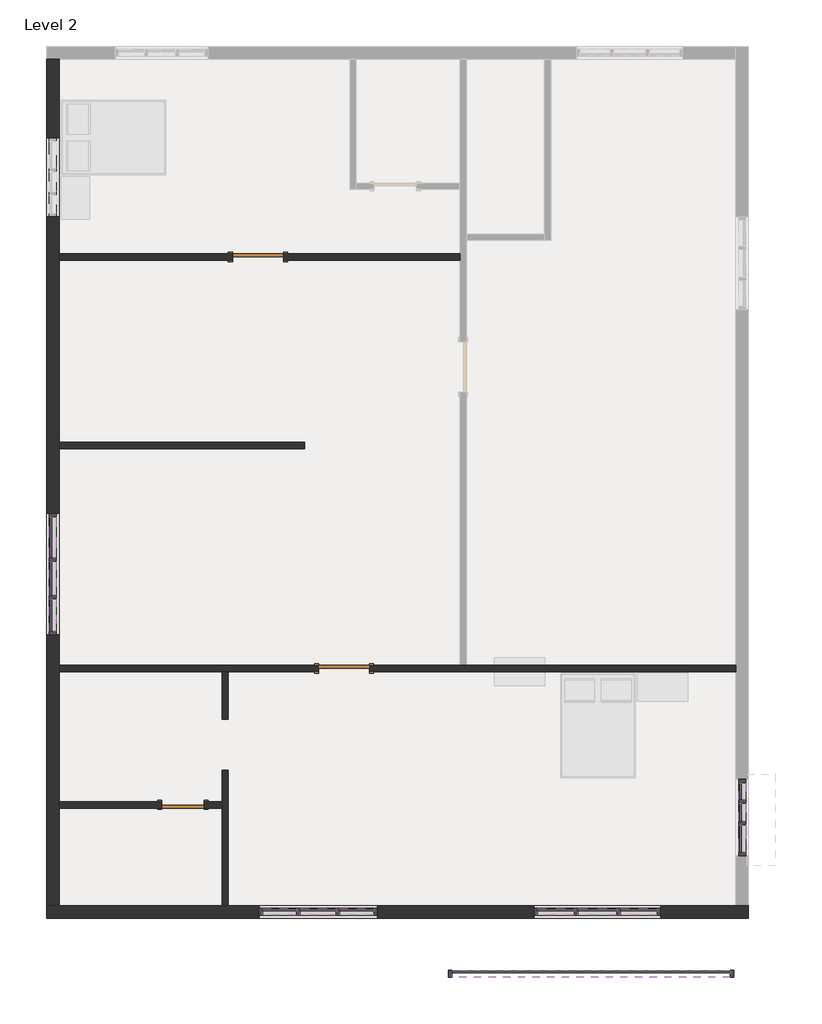
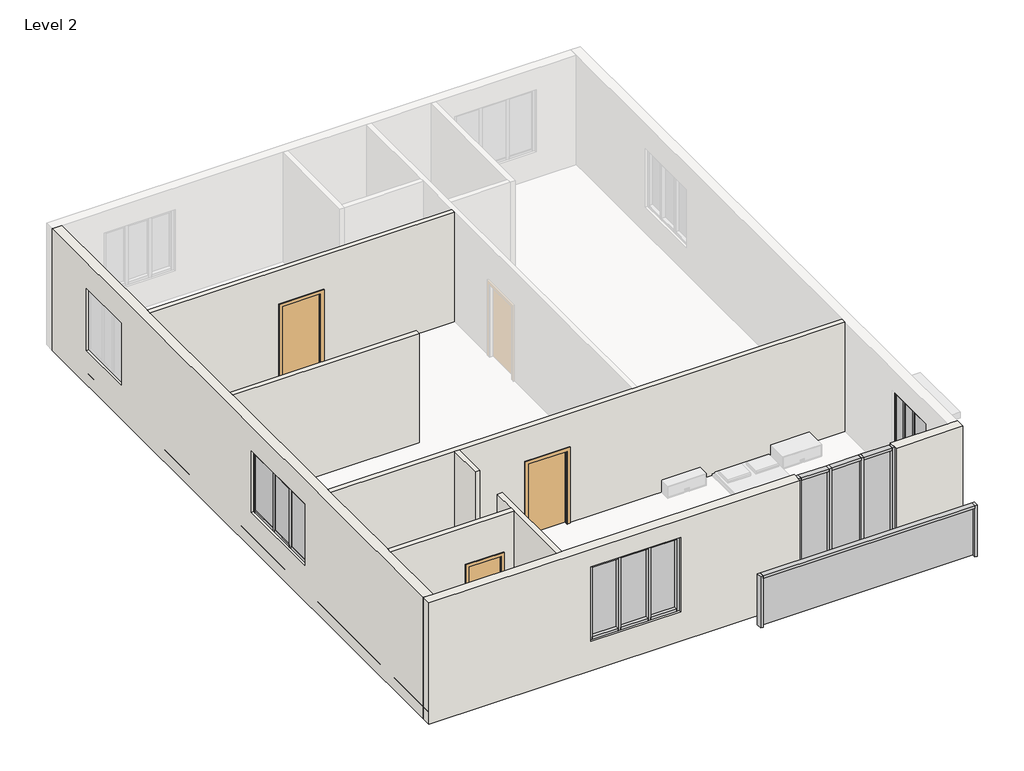
# One storey, part 1 of 2: 43 members, 13 plates, 8 walls, 3 doors.
"""IFC4 building model written with IfcOpenShell, lengths in millimetres."""

from ifc_helpers import new_model, si_unit, frame, origin, place, context, project, spatial, polyline, outline, extrude, faceted_brep, transform, mapped, element, save
from components import door_f2b275c1, door_e5f9f3c4, member_3f0e0172, member_5215b92c, member_ff9f2d30, member_780abd71, member_719f051b, member_c33c434a, member_b955a9e9, member_5fae7eaf, member_bd9e6ea3, member_b9f3750b, member_e45318c1, member_83289212, member_8199a1f0, member_b79e7e47, member_0fdf3d9d, member_3a0a7659, member_b984fe7d, member_72fd50dd, member_54cb9db3, member_9fca3acb, system_panel_glazed_d85bf7d9, system_panel_glazed_64df1ed2, system_panel_glazed_4d630f51, system_panel_glazed_9b1662f5, system_panel_glazed_97e07e6e, system_panel_glazed_53ed24d2, system_panel_glazed_8a1f71ef, system_panel_glazed_7c7839b8, system_panel_glazed_14be1180, system_panel_glazed_4048e9f5, system_panel_glazed_0f7bc74d

model = new_model("IFC4")

# Units and contexts
model_context = context("Model", 3, world=origin())
ifc_project = project(units=[si_unit("LENGTHUNIT", "METRE", prefix="MILLI")], contexts=[model_context])

# Site, building, storey
site = spatial("IfcSite", under=ifc_project)
building = spatial("IfcBuilding", under=site)
storey = spatial("IfcBuildingStorey", under=building, Name="Level 2", Elevation=3048.0)

# Doors
placement = place(None, origin())
door_shape = door_f2b275c1(model_context)
element("IfcDoor", 1, ObjectType="Single-Flush : 30\" x 80\"", at=placement, inside=storey, context=model_context, shape_type="MappedRepresentation", body=[
    mapped(door_shape, transform((-21008.0886697, -10163.1261954, 3048.0), x_axis=(1.0, 0.0, 0.0), y_axis=(0.0, 1.0, 0.0), z_axis=(0.0, 0.0, 1.0))),
])
door_2_shape = door_e5f9f3c4(model_context)
element("IfcDoor", 2, ObjectType="Single-Flush : 36\" x 84\"", at=placement, inside=storey, context=model_context, shape_type="MappedRepresentation", body=[
    mapped(door_2_shape, transform((-19655.5386697, -298.4011954, 3048.0), x_axis=(1.0, 0.0, 0.0), y_axis=(0.0, 1.0, 0.0), z_axis=(0.0, 0.0, 1.0))),
])
element("IfcDoor", 3, ObjectType="Single-Flush : 36\" x 84\"", at=placement, inside=storey, context=model_context, shape_type="MappedRepresentation", body=[
    mapped(door_2_shape, transform((-18102.9636697, -7708.8511954, 3048.0), x_axis=(1.0, 0.0, 0.0), y_axis=(0.0, 1.0, 0.0), z_axis=(0.0, 0.0, 1.0))),
])

# Members
member_shape = member_3f0e0172(model_context)
element("IfcMember", 4, ObjectType="Rectangular Mullion : 2.5\" x 5\" rectangular", at=placement, inside=storey, context=model_context, shape_type="MappedRepresentation", body=[
    mapped(member_shape, transform((-18957.0386697, -12090.3511954, 5652.7789545), x_axis=(0.0, 0.0, 1.0), y_axis=(0.0, -1.0, 0.0), z_axis=(1.0, 0.0, 0.0))),
])
element("IfcMember", 5, ObjectType="Rectangular Mullion : 2.5\" x 5\" rectangular", at=placement, inside=storey, context=model_context, shape_type="MappedRepresentation", body=[
    mapped(member_shape, transform((-17566.3886697, -12090.3511954, 5652.7789545), x_axis=(0.0, 0.0, 1.0), y_axis=(0.0, -1.0, 0.0), z_axis=(1.0, 0.0, 0.0))),
])
element("IfcMember", 6, ObjectType="Rectangular Mullion : 2.5\" x 5\" rectangular", at=placement, inside=storey, context=model_context, shape_type="MappedRepresentation", body=[
    mapped(member_shape, transform((-18182.3386697, -12090.3511954, 3784.7260489), x_axis=(0.0, 0.0, -1.0), y_axis=(0.0, -1.0, 0.0), z_axis=(-1.0, 0.0, 0.0))),
])
element("IfcMember", 7, ObjectType="Rectangular Mullion : 2.5\" x 5\" rectangular", at=placement, inside=storey, context=model_context, shape_type="MappedRepresentation", body=[
    mapped(member_shape, transform((-19572.9886697, -12090.3511954, 3784.7260489), x_axis=(0.0, 0.0, -1.0), y_axis=(0.0, -1.0, 0.0), z_axis=(-1.0, 0.0, 0.0))),
])
member_2_shape = member_5215b92c(model_context)
element("IfcMember", 8, ObjectType="Rectangular Mullion : 2.5\" x 5\" rectangular", at=placement, inside=storey, context=model_context, shape_type="MappedRepresentation", body=[
    mapped(member_2_shape, transform((-18245.8386697, -12090.3511954, 5652.7789545), x_axis=(0.0, 0.0, 1.0), y_axis=(0.0, -1.0, 0.0), z_axis=(1.0, 0.0, 0.0))),
])
element("IfcMember", 9, ObjectType="Rectangular Mullion : 2.5\" x 5\" rectangular", at=placement, inside=storey, context=model_context, shape_type="MappedRepresentation", body=[
    mapped(member_2_shape, transform((-18893.5386697, -12090.3511954, 3784.7260489), x_axis=(0.0, 0.0, -1.0), y_axis=(0.0, -1.0, 0.0), z_axis=(-1.0, 0.0, 0.0))),
])
member_3_shape = member_ff9f2d30(model_context)
element("IfcMember", 10, ObjectType="Rectangular Mullion : 2.5\" x 5\" rectangular", at=placement, inside=storey, context=model_context, shape_type="MappedRepresentation", body=[
    mapped(member_3_shape, transform((-10930.6386697, -10461.5761954, 4038.9192224), x_axis=(0.0, 0.0, -1.0), y_axis=(1.0, 0.0, 0.0), z_axis=(0.0, -1.0, 0.0))),
])
element("IfcMember", 11, ObjectType="Rectangular Mullion : 2.5\" x 5\" rectangular", at=placement, inside=storey, context=model_context, shape_type="MappedRepresentation", body=[
    mapped(member_3_shape, transform((-10930.6386697, -10131.3761954, 5551.780974), x_axis=(0.0, 0.0, 1.0), y_axis=(1.0, 0.0, 0.0), z_axis=(0.0, 1.0, 0.0))),
])
member_4_shape = member_780abd71(model_context)
element("IfcMember", 12, ObjectType="Rectangular Mullion : 2.5\" x 5\" rectangular", at=placement, inside=storey, context=model_context, shape_type="MappedRepresentation", body=[
    mapped(member_4_shape, transform((-18925.2886697, -12090.3511954, 3784.7260489), x_axis=(1.0, 0.0, 0.0), y_axis=(0.0, -1.0, 0.0), z_axis=(0.0, 0.0, -1.0))),
])
element("IfcMember", 13, ObjectType="Rectangular Mullion : 2.5\" x 5\" rectangular", at=placement, inside=storey, context=model_context, shape_type="MappedRepresentation", body=[
    mapped(member_4_shape, transform((-18214.0886697, -12090.3511954, 3784.7260489), x_axis=(1.0, 0.0, 0.0), y_axis=(0.0, -1.0, 0.0), z_axis=(0.0, 0.0, -1.0))),
])
member_5_shape = member_719f051b(model_context)
element("IfcMember", 14, ObjectType="Rectangular Mullion : 2.5\" x 5\" rectangular", at=placement, inside=storey, context=model_context, shape_type="MappedRepresentation", body=[
    mapped(member_5_shape, transform((-19636.4886697, -12090.3511954, 5652.7789545), x_axis=(-1.0, 0.0, 0.0), y_axis=(0.0, -1.0, 0.0), z_axis=(0.0, 0.0, 1.0))),
])
element("IfcMember", 15, ObjectType="Rectangular Mullion : 2.5\" x 5\" rectangular", at=placement, inside=storey, context=model_context, shape_type="MappedRepresentation", body=[
    mapped(member_5_shape, transform((-17502.8886697, -12090.3511954, 3784.7260489), x_axis=(1.0, 0.0, 0.0), y_axis=(0.0, -1.0, 0.0), z_axis=(0.0, 0.0, -1.0))),
])
member_6_shape = member_c33c434a(model_context)
element("IfcMember", 16, ObjectType="Rectangular Mullion : 2.5\" x 5\" rectangular", at=placement, inside=storey, context=model_context, shape_type="MappedRepresentation", body=[
    mapped(member_6_shape, transform((-13953.2386697, -12090.3511954, 6096.0), x_axis=(0.0, 0.0, 1.0), y_axis=(0.0, -1.0, 0.0), z_axis=(1.0, 0.0, 0.0))),
])
element("IfcMember", 17, ObjectType="Rectangular Mullion : 2.5\" x 5\" rectangular", at=placement, inside=storey, context=model_context, shape_type="MappedRepresentation", body=[
    mapped(member_6_shape, transform((-12460.9886697, -12090.3511954, 6096.0), x_axis=(0.0, 0.0, 1.0), y_axis=(0.0, -1.0, 0.0), z_axis=(1.0, 0.0, 0.0))),
])
member_7_shape = member_b955a9e9(model_context)
element("IfcMember", 18, ObjectType="Rectangular Mullion : 2.5\" x 5\" rectangular", at=placement, inside=storey, context=model_context, shape_type="MappedRepresentation", body=[
    mapped(member_7_shape, transform((-13191.2386697, -12090.3511954, 6096.0), x_axis=(0.0, 0.0, 1.0), y_axis=(0.0, -1.0, 0.0), z_axis=(1.0, 0.0, 0.0))),
])
member_8_shape = member_5fae7eaf(model_context)
element("IfcMember", 19, ObjectType="Rectangular Mullion : 2.5\" x 5\" rectangular", at=placement, inside=storey, context=model_context, shape_type="MappedRepresentation", body=[
    mapped(member_8_shape, transform((-13921.4886697, -12090.3511954, 3684.4190385), x_axis=(1.0, 0.0, 0.0), y_axis=(0.0, -1.0, 0.0), z_axis=(0.0, 0.0, -1.0))),
])
element("IfcMember", 20, ObjectType="Rectangular Mullion : 2.5\" x 5\" rectangular", at=placement, inside=storey, context=model_context, shape_type="MappedRepresentation", body=[
    mapped(member_8_shape, transform((-13159.4886697, -12090.3511954, 3684.4190385), x_axis=(1.0, 0.0, 0.0), y_axis=(0.0, -1.0, 0.0), z_axis=(0.0, 0.0, -1.0))),
])
element("IfcMember", 21, ObjectType="Rectangular Mullion : 2.5\" x 5\" rectangular", at=placement, inside=storey, context=model_context, shape_type="MappedRepresentation", body=[
    mapped(member_6_shape, transform((-13127.7386697, -12090.3511954, 3684.4190385), x_axis=(0.0, 0.0, -1.0), y_axis=(0.0, -1.0, 0.0), z_axis=(-1.0, 0.0, 0.0))),
])
element("IfcMember", 22, ObjectType="Rectangular Mullion : 2.5\" x 5\" rectangular", at=placement, inside=storey, context=model_context, shape_type="MappedRepresentation", body=[
    mapped(member_6_shape, transform((-14619.9886697, -12090.3511954, 3684.4190385), x_axis=(0.0, 0.0, -1.0), y_axis=(0.0, -1.0, 0.0), z_axis=(-1.0, 0.0, 0.0))),
])
element("IfcMember", 23, ObjectType="Rectangular Mullion : 2.5\" x 5\" rectangular", at=placement, inside=storey, context=model_context, shape_type="MappedRepresentation", body=[
    mapped(member_7_shape, transform((-13889.7386697, -12090.3511954, 3684.4190385), x_axis=(0.0, 0.0, -1.0), y_axis=(0.0, -1.0, 0.0), z_axis=(-1.0, 0.0, 0.0))),
])
member_9_shape = member_bd9e6ea3(model_context)
element("IfcMember", 24, ObjectType="Rectangular Mullion : 2.5\" x 5\" rectangular", at=placement, inside=storey, context=model_context, shape_type="MappedRepresentation", body=[
    mapped(member_9_shape, transform((-14683.4886697, -12090.3511954, 6096.0), x_axis=(-1.0, 0.0, 0.0), y_axis=(0.0, -1.0, 0.0), z_axis=(0.0, 0.0, 1.0))),
])
element("IfcMember", 25, ObjectType="Rectangular Mullion : 2.5\" x 5\" rectangular", at=placement, inside=storey, context=model_context, shape_type="MappedRepresentation", body=[
    mapped(member_9_shape, transform((-12397.4886697, -12090.3511954, 3684.4190385), x_axis=(1.0, 0.0, 0.0), y_axis=(0.0, -1.0, 0.0), z_axis=(0.0, 0.0, -1.0))),
])
member_10_shape = member_b9f3750b(model_context)
element("IfcMember", 26, ObjectType="Rectangular Mullion : 2.5\" x 5\" rectangular", at=placement, inside=storey, context=model_context, shape_type="MappedRepresentation", body=[
    mapped(member_10_shape, transform((-10930.6386697, -10525.0761954, 5551.780974), x_axis=(0.0, 0.0, 1.0), y_axis=(1.0, 0.0, 0.0), z_axis=(0.0, 1.0, 0.0))),
])
member_11_shape = member_e45318c1(model_context)
element("IfcMember", 27, ObjectType="Rectangular Mullion : 2.5\" x 5\" rectangular", at=placement, inside=storey, context=model_context, shape_type="MappedRepresentation", body=[
    mapped(member_11_shape, transform((-10930.6386697, -10099.6261954, 4038.9192224), x_axis=(0.0, 1.0, 0.0), y_axis=(1.0, 0.0, 0.0), z_axis=(0.0, 0.0, -1.0))),
])
element("IfcMember", 28, ObjectType="Rectangular Mullion : 2.5\" x 5\" rectangular", at=placement, inside=storey, context=model_context, shape_type="MappedRepresentation", body=[
    mapped(member_11_shape, transform((-10930.6386697, -10493.3261954, 4038.9192224), x_axis=(0.0, 1.0, 0.0), y_axis=(1.0, 0.0, 0.0), z_axis=(0.0, 0.0, -1.0))),
])
element("IfcMember", 29, ObjectType="Rectangular Mullion : 2.5\" x 5\" rectangular", at=placement, inside=storey, context=model_context, shape_type="MappedRepresentation", body=[
    mapped(member_10_shape, transform((-10930.6386697, -11014.0261954, 4038.9192224), x_axis=(0.0, 0.0, -1.0), y_axis=(1.0, 0.0, 0.0), z_axis=(0.0, -1.0, 0.0))),
])
member_12_shape = member_83289212(model_context)
element("IfcMember", 30, ObjectType="Rectangular Mullion : 2.5\" x 5\" rectangular", at=placement, inside=storey, context=model_context, shape_type="MappedRepresentation", body=[
    mapped(member_12_shape, transform((-10930.6386697, -11077.5261954, 5551.780974), x_axis=(0.0, -1.0, 0.0), y_axis=(1.0, 0.0, 0.0), z_axis=(0.0, 0.0, 1.0))),
])
member_13_shape = member_8199a1f0(model_context)
element("IfcMember", 31, ObjectType="Rectangular Mullion : 2.5\" x 5\" rectangular", at=placement, inside=storey, context=model_context, shape_type="MappedRepresentation", body=[
    mapped(member_13_shape, transform((-10930.6386697, -9769.4261954, 5551.780974), x_axis=(0.0, 0.0, 1.0), y_axis=(1.0, 0.0, 0.0), z_axis=(0.0, 1.0, 0.0))),
])
element("IfcMember", 32, ObjectType="Rectangular Mullion : 2.5\" x 5\" rectangular", at=placement, inside=storey, context=model_context, shape_type="MappedRepresentation", body=[
    mapped(member_13_shape, transform((-10930.6386697, -10067.8761954, 4038.9192224), x_axis=(0.0, 0.0, -1.0), y_axis=(1.0, 0.0, 0.0), z_axis=(0.0, -1.0, 0.0))),
])
element("IfcMember", 33, ObjectType="Rectangular Mullion : 2.5\" x 5\" rectangular", at=placement, inside=storey, context=model_context, shape_type="MappedRepresentation", body=[
    mapped(member_12_shape, transform((-10930.6386697, -9705.9261954, 4038.9192224), x_axis=(0.0, 1.0, 0.0), y_axis=(1.0, 0.0, 0.0), z_axis=(0.0, 0.0, -1.0))),
])
member_14_shape = member_b79e7e47(model_context)
element("IfcMember", 34, ObjectType="Rectangular Mullion : 2.5\" x 5\" rectangular", at=placement, inside=storey, context=model_context, shape_type="MappedRepresentation", body=[
    mapped(member_14_shape, transform((-23351.2386697, -6454.7261954, 5474.6486322), x_axis=(0.0, 0.0, 1.0), y_axis=(1.0, 0.0, 0.0), z_axis=(0.0, 1.0, 0.0))),
])
member_15_shape = member_0fdf3d9d(model_context)
element("IfcMember", 35, ObjectType="Rectangular Mullion : 2.5\" x 5\" rectangular", at=placement, inside=storey, context=model_context, shape_type="MappedRepresentation", body=[
    mapped(member_15_shape, transform((-23351.2386697, -5778.4511954, 5474.6486322), x_axis=(0.0, 0.0, 1.0), y_axis=(1.0, 0.0, 0.0), z_axis=(0.0, 1.0, 0.0))),
])
member_16_shape = member_3a0a7659(model_context)
element("IfcMember", 36, ObjectType="Rectangular Mullion : 2.5\" x 5\" rectangular", at=placement, inside=storey, context=model_context, shape_type="MappedRepresentation", body=[
    mapped(member_16_shape, transform((-23351.2386697, -4972.0011954, 5474.6486322), x_axis=(0.0, 0.0, 1.0), y_axis=(1.0, 0.0, 0.0), z_axis=(0.0, 1.0, 0.0))),
])
member_17_shape = member_b984fe7d(model_context)
element("IfcMember", 37, ObjectType="Rectangular Mullion : 2.5\" x 5\" rectangular", at=placement, inside=storey, context=model_context, shape_type="MappedRepresentation", body=[
    mapped(member_17_shape, transform((-23351.2386697, -5746.7011954, 3943.3117705), x_axis=(0.0, 1.0, 0.0), y_axis=(1.0, 0.0, 0.0), z_axis=(0.0, 0.0, -1.0))),
])
element("IfcMember", 38, ObjectType="Rectangular Mullion : 2.5\" x 5\" rectangular", at=placement, inside=storey, context=model_context, shape_type="MappedRepresentation", body=[
    mapped(member_17_shape, transform((-23351.2386697, -6422.9761954, 3943.3117705), x_axis=(0.0, 1.0, 0.0), y_axis=(1.0, 0.0, 0.0), z_axis=(0.0, 0.0, -1.0))),
])
element("IfcMember", 39, ObjectType="Rectangular Mullion : 2.5\" x 5\" rectangular", at=placement, inside=storey, context=model_context, shape_type="MappedRepresentation", body=[
    mapped(member_15_shape, transform((-23351.2386697, -6391.2261954, 3943.3117705), x_axis=(0.0, 0.0, -1.0), y_axis=(1.0, 0.0, 0.0), z_axis=(0.0, -1.0, 0.0))),
])
element("IfcMember", 40, ObjectType="Rectangular Mullion : 2.5\" x 5\" rectangular", at=placement, inside=storey, context=model_context, shape_type="MappedRepresentation", body=[
    mapped(member_16_shape, transform((-23351.2386697, -5714.9511954, 3943.3117705), x_axis=(0.0, 0.0, -1.0), y_axis=(1.0, 0.0, 0.0), z_axis=(0.0, -1.0, 0.0))),
])
element("IfcMember", 41, ObjectType="Rectangular Mullion : 2.5\" x 5\" rectangular", at=placement, inside=storey, context=model_context, shape_type="MappedRepresentation", body=[
    mapped(member_14_shape, transform((-23351.2386697, -7035.7511954, 3943.3117705), x_axis=(0.0, 0.0, -1.0), y_axis=(1.0, 0.0, 0.0), z_axis=(0.0, -1.0, 0.0))),
])
member_18_shape = member_72fd50dd(model_context)
element("IfcMember", 42, ObjectType="Rectangular Mullion : 2.5\" x 5\" rectangular", at=placement, inside=storey, context=model_context, shape_type="MappedRepresentation", body=[
    mapped(member_18_shape, transform((-23351.2386697, -7099.2511954, 5474.6486322), x_axis=(0.0, -1.0, 0.0), y_axis=(1.0, 0.0, 0.0), z_axis=(0.0, 0.0, 1.0))),
])
element("IfcMember", 43, ObjectType="Rectangular Mullion : 2.5\" x 5\" rectangular", at=placement, inside=storey, context=model_context, shape_type="MappedRepresentation", body=[
    mapped(member_18_shape, transform((-23351.2386697, -4908.5011954, 3943.3117705), x_axis=(0.0, 1.0, 0.0), y_axis=(1.0, 0.0, 0.0), z_axis=(0.0, 0.0, -1.0))),
])
member_19_shape = member_54cb9db3(model_context)
element("IfcMember", 44, ObjectType="Rectangular Mullion : 2.5\" x 5\" rectangular", at=placement, inside=storey, context=model_context, shape_type="MappedRepresentation", body=[
    mapped(member_19_shape, transform((-16224.7214825, -13207.9511954, 4860.1647633), x_axis=(-1.0, 0.0, 0.0), y_axis=(0.0, -1.0, 0.0), z_axis=(0.0, 0.0, 1.0))),
])
member_20_shape = member_9fca3acb(model_context)
element("IfcMember", 45, ObjectType="Rectangular Mullion : 2.5\" x 5\" rectangular", at=placement, inside=storey, context=model_context, shape_type="MappedRepresentation", body=[
    mapped(member_20_shape, transform((-11147.6908348, -13207.9511954, 4860.1647633), x_axis=(0.0, 0.0, 1.0), y_axis=(0.0, -1.0, 0.0), z_axis=(1.0, 0.0, 0.0))),
])
element("IfcMember", 46, ObjectType="Rectangular Mullion : 2.5\" x 5\" rectangular", at=placement, inside=storey, context=model_context, shape_type="MappedRepresentation", body=[
    mapped(member_19_shape, transform((-11084.1908348, -13207.9511954, 3577.3120422), x_axis=(1.0, 0.0, 0.0), y_axis=(0.0, -1.0, 0.0), z_axis=(0.0, 0.0, -1.0))),
])

# Plates
system_panel_glazed_shape = system_panel_glazed_d85bf7d9(model_context)
element("IfcPlate", 47, ObjectType="System Panel : Glazed", at=placement, inside=storey, context=model_context, shape_type="MappedRepresentation", body=[
    mapped(system_panel_glazed_shape, transform((-19265.0136697, -12090.3511954, 3848.2260489), x_axis=(1.0, 0.0, 0.0), y_axis=(0.0, 1.0, 0.0), z_axis=(0.0, 0.0, 1.0))),
])
element("IfcPlate", 48, ObjectType="System Panel : Glazed", at=placement, inside=storey, context=model_context, shape_type="MappedRepresentation", body=[
    mapped(system_panel_glazed_shape, transform((-17874.3636697, -12090.3511954, 3848.2260489), x_axis=(1.0, 0.0, 0.0), y_axis=(0.0, 1.0, 0.0), z_axis=(0.0, 0.0, 1.0))),
])
system_panel_glazed_2_shape = system_panel_glazed_64df1ed2(model_context)
element("IfcPlate", 49, ObjectType="System Panel : Glazed", at=placement, inside=storey, context=model_context, shape_type="MappedRepresentation", body=[
    mapped(system_panel_glazed_2_shape, transform((-18569.6886697, -12090.3511954, 3848.2260489), x_axis=(1.0, 0.0, 0.0), y_axis=(0.0, 1.0, 0.0), z_axis=(0.0, 0.0, 1.0))),
])
system_panel_glazed_3_shape = system_panel_glazed_4d630f51(model_context)
element("IfcPlate", 50, ObjectType="System Panel : Glazed", at=placement, inside=storey, context=model_context, shape_type="MappedRepresentation", body=[
    mapped(system_panel_glazed_3_shape, transform((-14286.6136697, -12090.3511954, 3747.9190385), x_axis=(1.0, 0.0, 0.0), y_axis=(0.0, 1.0, 0.0), z_axis=(0.0, 0.0, 1.0))),
])
element("IfcPlate", 51, ObjectType="System Panel : Glazed", at=placement, inside=storey, context=model_context, shape_type="MappedRepresentation", body=[
    mapped(system_panel_glazed_3_shape, transform((-12794.3636697, -12090.3511954, 3747.9190385), x_axis=(1.0, 0.0, 0.0), y_axis=(0.0, 1.0, 0.0), z_axis=(0.0, 0.0, 1.0))),
])
system_panel_glazed_4_shape = system_panel_glazed_9b1662f5(model_context)
element("IfcPlate", 52, ObjectType="System Panel : Glazed", at=placement, inside=storey, context=model_context, shape_type="MappedRepresentation", body=[
    mapped(system_panel_glazed_4_shape, transform((-13540.4886697, -12090.3511954, 3747.9190385), x_axis=(1.0, 0.0, 0.0), y_axis=(0.0, 1.0, 0.0), z_axis=(0.0, 0.0, 1.0))),
])
system_panel_glazed_5_shape = system_panel_glazed_97e07e6e(model_context)
element("IfcPlate", 53, ObjectType="System Panel : Glazed", at=placement, inside=storey, context=model_context, shape_type="MappedRepresentation", body=[
    mapped(system_panel_glazed_5_shape, transform((-10930.6386697, -10769.5511954, 4102.4192224), x_axis=(0.0, 1.0, 0.0), y_axis=(-1.0, 0.0, 0.0), z_axis=(0.0, 0.0, 1.0))),
])
system_panel_glazed_6_shape = system_panel_glazed_53ed24d2(model_context)
element("IfcPlate", 54, ObjectType="System Panel : Glazed", at=placement, inside=storey, context=model_context, shape_type="MappedRepresentation", body=[
    mapped(system_panel_glazed_6_shape, transform((-10930.6386697, -10296.4761954, 4102.4192224), x_axis=(0.0, 1.0, 0.0), y_axis=(-1.0, 0.0, 0.0), z_axis=(0.0, 0.0, 1.0))),
])
system_panel_glazed_7_shape = system_panel_glazed_8a1f71ef(model_context)
element("IfcPlate", 55, ObjectType="System Panel : Glazed", at=placement, inside=storey, context=model_context, shape_type="MappedRepresentation", body=[
    mapped(system_panel_glazed_7_shape, transform((-10930.6386697, -9918.6511954, 4102.4192224), x_axis=(0.0, 1.0, 0.0), y_axis=(-1.0, 0.0, 0.0), z_axis=(0.0, 0.0, 1.0))),
])
system_panel_glazed_8_shape = system_panel_glazed_7c7839b8(model_context)
element("IfcPlate", 56, ObjectType="System Panel : Glazed", at=placement, inside=storey, context=model_context, shape_type="MappedRepresentation", body=[
    mapped(system_panel_glazed_8_shape, transform((-23351.2386697, -6745.2386954, 4006.8117705), x_axis=(0.0, 1.0, 0.0), y_axis=(-1.0, 0.0, 0.0), z_axis=(0.0, 0.0, 1.0))),
])
system_panel_glazed_9_shape = system_panel_glazed_14be1180(model_context)
element("IfcPlate", 57, ObjectType="System Panel : Glazed", at=placement, inside=storey, context=model_context, shape_type="MappedRepresentation", body=[
    mapped(system_panel_glazed_9_shape, transform((-23351.2386697, -5343.4761954, 4006.8117705), x_axis=(0.0, 1.0, 0.0), y_axis=(-1.0, 0.0, 0.0), z_axis=(0.0, 0.0, 1.0))),
])
system_panel_glazed_10_shape = system_panel_glazed_4048e9f5(model_context)
element("IfcPlate", 58, ObjectType="System Panel : Glazed", at=placement, inside=storey, context=model_context, shape_type="MappedRepresentation", body=[
    mapped(system_panel_glazed_10_shape, transform((-23351.2386697, -6084.8386954, 4006.8117705), x_axis=(0.0, 1.0, 0.0), y_axis=(-1.0, 0.0, 0.0), z_axis=(0.0, 0.0, 1.0))),
])
system_panel_glazed_11_shape = system_panel_glazed_0f7bc74d(model_context)
element("IfcPlate", 59, ObjectType="System Panel : Glazed", at=placement, inside=storey, context=model_context, shape_type="MappedRepresentation", body=[
    mapped(system_panel_glazed_11_shape, transform((-13654.4561587, -13207.9511954, 3577.3120422), x_axis=(1.0, 0.0, 0.0), y_axis=(0.0, 1.0, 0.0), z_axis=(0.0, 0.0, 1.0))),
])

# Walls
element("IfcWall", 60, ObjectType="4.5\"", at=placement, inside=storey, context=model_context, shape_type="Brep", body=[
    faceted_brep([(-20188.9386697, -11976.0511954, 3048.0), (-20188.9386697, -9537.6511954, 3048.0), (-20188.9386697, -9537.6511954, 6096.0), (-20188.9386697, -11976.0511954, 6096.0), (-20303.2386697, -11976.0511954, 3048.0), (-20303.2386697, -11976.0511954, 6096.0), (-20303.2386697, -10220.2761954, 6096.0), (-20303.2386697, -10105.9761954, 6096.0), (-20303.2386697, -9537.6511954, 6096.0), (-20303.2386697, -9537.6511954, 3048.0), (-20303.2386697, -10105.9761954, 3048.0), (-20303.2386697, -10220.2761954, 3048.0)], [[[0, 1, 2, 3]], [[4, 5, 6, 7, 8, 9, 10, 11]], [[1, 0, 4, 11, 10, 9]], [[2, 1, 9, 8]], [[3, 2, 8, 7, 6, 5]], [[0, 3, 5, 4]]]),
])
element("IfcWall", 61, ObjectType="4.5\"", at=placement, inside=storey, context=model_context, shape_type="Brep", body=[
    faceted_brep([(-11044.9386697, -7651.7011954, 3048.0), (-15902.6886697, -7651.7011954, 3048.0), (-16016.9886697, -7651.7011954, 3048.0), (-17645.7636697, -7651.7011954, 3048.0), (-17645.7636697, -7651.7011954, 5181.6), (-18560.1636697, -7651.7011954, 5181.6), (-18560.1636697, -7651.7011954, 3048.0), (-23236.9386697, -7651.7011954, 3048.0), (-23236.9386697, -7651.7011954, 6096.0), (-16016.9886697, -7651.7011954, 6096.0), (-15902.6886697, -7651.7011954, 6096.0), (-11044.9386697, -7651.7011954, 6096.0), (-17645.7636697, -7766.0011954, 5181.6), (-17645.7636697, -7766.0011954, 3048.0), (-11044.9386697, -7766.0011954, 3048.0), (-11044.9386697, -7766.0011954, 6096.0), (-20188.9386697, -7766.0011954, 6096.0), (-20303.2386697, -7766.0011954, 6096.0), (-23236.9386697, -7766.0011954, 6096.0), (-23236.9386697, -7766.0011954, 3048.0), (-20303.2386697, -7766.0011954, 3048.0), (-20188.9386697, -7766.0011954, 3048.0), (-18560.1636697, -7766.0011954, 3048.0), (-18560.1636697, -7766.0011954, 5181.6)], [[[0, 1, 2, 3, 4, 5, 6, 7, 8, 9, 10, 11]], [[12, 13, 14, 15, 16, 17, 18, 19, 20, 21, 22, 23]], [[14, 13, 3, 2, 1, 0]], [[22, 21, 20, 19, 7, 6]], [[11, 10, 9, 8, 18, 17, 16, 15]], [[8, 7, 19, 18]], [[0, 11, 15, 14]], [[4, 3, 13, 12]], [[5, 4, 12, 23]], [[6, 5, 23, 22]]]),
])
element("IfcWall", 62, ObjectType="4.5\"", at=placement, inside=storey, context=model_context, shape_type="SweptSolid", body=[
    extrude(outline(polyline([(5080.0, -20627.0886697), (3048.0, -20627.0886697), (3048.0, -20303.2386697), (6096.0, -20303.2386697), (6096.0, -23236.9386697), (3048.0, -23236.9386697), (3048.0, -21389.0886697), (5080.0, -21389.0886697), (5080.0, -20627.0886697)])), frame((0.0, -10220.2761954, 0.0), z_axis=(0.0, 1.0, 0.0), x_axis=(0.0, 0.0, 1.0)), (0.0, 0.0, 1.0), 114.3),
])
element("IfcWall", 63, ObjectType="4.5\"", at=placement, inside=storey, context=model_context, shape_type="SweptSolid", body=[
    extrude(outline(polyline([(5181.6, -19198.3386697), (3048.0, -19198.3386697), (3048.0, -16016.9886697), (6096.0, -16016.9886697), (6096.0, -23236.9386697), (3048.0, -23236.9386697), (3048.0, -20112.7386697), (5181.6, -20112.7386697), (5181.6, -19198.3386697)])), frame((0.0, -355.5511954, 0.0), z_axis=(0.0, 1.0, 0.0), x_axis=(0.0, 0.0, 1.0)), (0.0, 0.0, 1.0), 114.3),
])
element("IfcWall", 64, ObjectType="4.5\"", at=placement, inside=storey, context=model_context, shape_type="SweptSolid", body=[
    extrude(outline(polyline([(-18817.3386697, -3746.4511954), (-23236.9386697, -3746.4511954), (-23236.9386697, -3632.1511954), (-18817.3386697, -3632.1511954), (-18817.3386697, -3746.4511954)])), frame((0.0, 0.0, 3048.0), z_axis=(0.0, 0.0, 1.0), x_axis=(1.0, 0.0, 0.0)), (0.0, 0.0, 1.0), 3048.0),
])
element("IfcWall", 65, ObjectType="4.5\"", at=placement, inside=storey, context=model_context, shape_type="SweptSolid", body=[
    extrude(outline(polyline([(-20188.9386697, -7766.0011954), (-20188.9386697, -8623.2511954), (-20303.2386697, -8623.2511954), (-20303.2386697, -7766.0011954), (-20188.9386697, -7766.0011954)])), frame((0.0, 0.0, 3048.0), z_axis=(0.0, 0.0, 1.0), x_axis=(1.0, 0.0, 0.0)), (0.0, 0.0, 1.0), 3048.0),
])
element("IfcWall", 66, ObjectType="9\"", at=placement, inside=storey, context=model_context, shape_type="Brep", body=[
    faceted_brep([(-23465.5386697, -12204.6511954, 3048.0), (-10816.3386697, -12204.6511954, 3048.0), (-10816.3386697, -12204.6511954, 6096.0), (-12397.4886697, -12204.6511954, 6096.0), (-12397.4886697, -12204.6511954, 3684.4190385), (-14683.4886697, -12204.6511954, 3684.4190385), (-14683.4886697, -12204.6511954, 6096.0), (-23465.5386697, -12204.6511954, 6096.0), (-19636.4886697, -12204.6511954, 3784.7260489), (-19636.4886697, -12204.6511954, 5652.7789545), (-17502.8886697, -12204.6511954, 5652.7789545), (-17502.8886697, -12204.6511954, 3784.7260489), (-10816.3386697, -11976.0511954, 3048.0), (-11044.9386697, -11976.0511954, 3048.0), (-20188.9386697, -11976.0511954, 3048.0), (-20303.2386697, -11976.0511954, 3048.0), (-23236.9386697, -11976.0511954, 3048.0), (-23465.5386697, -11976.0511954, 3048.0), (-23465.5386697, -11976.0511954, 6096.0), (-23236.9386697, -11976.0511954, 6096.0), (-20303.2386697, -11976.0511954, 6096.0), (-20188.9386697, -11976.0511954, 6096.0), (-14683.4886697, -11976.0511954, 6096.0), (-14683.4886697, -11976.0511954, 3684.4190385), (-12397.4886697, -11976.0511954, 3684.4190385), (-12397.4886697, -11976.0511954, 6096.0), (-11044.9386697, -11976.0511954, 6096.0), (-10816.3386697, -11976.0511954, 6096.0), (-19636.4886697, -11976.0511954, 5652.7789545), (-19636.4886697, -11976.0511954, 3784.7260489), (-17502.8886697, -11976.0511954, 3784.7260489), (-17502.8886697, -11976.0511954, 5652.7789545)], [[[0, 1, 2, 3, 4, 5, 6, 7], [8, 9, 10, 11]], [[12, 13, 14, 15, 16, 17, 18, 19, 20, 21, 22, 23, 24, 25, 26, 27], [28, 29, 30, 31]], [[1, 0, 17, 16, 15, 14, 13, 12]], [[2, 27, 26, 25, 3]], [[18, 7, 6, 22, 21, 20, 19]], [[2, 1, 12, 27]], [[0, 7, 18, 17]], [[8, 29, 28, 9]], [[9, 28, 31, 10]], [[10, 31, 30, 11]], [[29, 8, 11, 30]], [[5, 23, 22, 6]], [[24, 4, 3, 25]], [[23, 5, 4, 24]]]),
])
element("IfcWall", 67, ObjectType="9\"", at=placement, inside=storey, context=model_context, shape_type="Brep", body=[
    faceted_brep([(-23465.5386697, 3263.9488046, 3048.0), (-23465.5386697, -11976.0511954, 3048.0), (-23465.5386697, -11976.0511954, 6096.0), (-23465.5386697, 3263.9488046, 6096.0), (-23465.5386697, -7099.2511954, 5474.6486322), (-23465.5386697, -7099.2511954, 3943.3117705), (-23465.5386697, -4908.5011954, 3943.3117705), (-23465.5386697, -4908.5011954, 5474.6486322), (-23465.5386697, 425.4988046, 5453.2250414), (-23465.5386697, 425.4988046, 3896.5069058), (-23465.5386697, 1854.2488046, 3896.5069058), (-23465.5386697, 1854.2488046, 5453.2250414), (-23236.9386697, -11976.0511954, 3048.0), (-23236.9386697, -10220.2761954, 3048.0), (-23236.9386697, -10105.9761954, 3048.0), (-23236.9386697, -7766.0011954, 3048.0), (-23236.9386697, -7651.7011954, 3048.0), (-23236.9386697, -3746.4511954, 3048.0), (-23236.9386697, -3632.1511954, 3048.0), (-23236.9386697, -355.5511954, 3048.0), (-23236.9386697, -241.2511954, 3048.0), (-23236.9386697, 3263.9488046, 3048.0), (-23236.9386697, 3263.9488046, 6096.0), (-23236.9386697, -241.2511954, 6096.0), (-23236.9386697, -355.5511954, 6096.0), (-23236.9386697, -3632.1511954, 6096.0), (-23236.9386697, -3746.4511954, 6096.0), (-23236.9386697, -7651.7011954, 6096.0), (-23236.9386697, -7766.0011954, 6096.0), (-23236.9386697, -10105.9761954, 6096.0), (-23236.9386697, -10220.2761954, 6096.0), (-23236.9386697, -11976.0511954, 6096.0), (-23236.9386697, -7099.2511954, 3943.3117705), (-23236.9386697, -7099.2511954, 5474.6486322), (-23236.9386697, -4908.5011954, 5474.6486322), (-23236.9386697, -4908.5011954, 3943.3117705), (-23236.9386697, 425.4988046, 3896.5069058), (-23236.9386697, 425.4988046, 5453.2250414), (-23236.9386697, 1854.2488046, 5453.2250414), (-23236.9386697, 1854.2488046, 3896.5069058)], [[[0, 1, 2, 3], [4, 5, 6, 7], [8, 9, 10, 11]], [[12, 13, 14, 15, 16, 17, 18, 19, 20, 21, 22, 23, 24, 25, 26, 27, 28, 29, 30, 31], [32, 33, 34, 35], [36, 37, 38, 39]], [[1, 0, 21, 20, 19, 18, 17, 16, 15, 14, 13, 12]], [[3, 2, 31, 30, 29, 28, 27, 26, 25, 24, 23, 22]], [[2, 1, 12, 31]], [[0, 3, 22, 21]], [[32, 5, 4, 33]], [[33, 4, 7, 34]], [[34, 7, 6, 35]], [[5, 32, 35, 6]], [[8, 37, 36, 9]], [[37, 8, 11, 38]], [[38, 11, 10, 39]], [[9, 36, 39, 10]]]),
])

save(model, "model.ifc")

# Revit data of these elements
# Type "Single-Flush : 30\" x 80\""
#   Type Mark = "5"
#   Construction Type Id = "MDOOR"
#   Assembly Code = "C1020"
#   Analytic Construction = "Metal"
#   Thickness = 0' - 2"
#   Heat Transfer Coefficient (U) = 0.651978 BTU/(h·ft²·°F)
#   Height = 6' - 8"
#   Trim Projection Ext = 0' - 1"
#   Trim Projection Int = 0' - 1"
#   Trim Width = 0' - 3"
#   Width = 2' - 6"
#   Define Thermal Properties by = 1
#   Define Thermal Properties by = 1
#   Door Material = Door - Panel
#   Frame Material = Door - Frame
#   Visual Light Transmittance = 0
#   Solar Heat Gain Coefficient = 0
#   Function = (empty or 0)
#   Wall Closure = (empty or 0)
# Type "Single-Flush : 36\" x 84\""
#   Type Mark = "1"
#   Construction Type Id = "MDOOR"
#   Assembly Code = "C1020"
#   Analytic Construction = "Metal"
#   Thickness = 0' - 2"
#   Heat Transfer Coefficient (U) = 0.651978 BTU/(h·ft²·°F)
#   Height = 7' - 0"
#   Trim Projection Ext = 0' - 1"
#   Trim Projection Int = 0' - 1"
#   Trim Width = 0' - 3"
#   Width = 3' - 0"
#   Define Thermal Properties by = 1
#   Define Thermal Properties by = 1
#   Door Material = Door - Panel
#   Frame Material = Door - Frame
#   Visual Light Transmittance = 0
#   Solar Heat Gain Coefficient = 0
#   Function = (empty or 0)
#   Wall Closure = (empty or 0)
# Type "Rectangular Mullion : 2.5\" x 5\" rectangular"
#   built-in parameter 1007304 = 0.416667 (stored number, unit not read)
#   built-in parameter 1007301 = 0.104167 (stored number, unit not read)
#   built-in parameter 1007300 = 0.104167 (stored number, unit not read)
# Type "System Panel : Glazed"
#   Construction Type Id = "GSP4R"
#   Analytic Construction = "1/8 in Pilkington single glazing"
#   Visual Light Transmittance = 0.9
#   Solar Heat Gain Coefficient = 0.86
#   Heat Transfer Coefficient (U) = 1.18115 BTU/(h·ft²·°F)
#   Define Thermal Properties by = 1
# Type "4.5\""
#   Assembly Code = "B2010"
#   Layers, outside or top first: 0' - 4 1/2" no material (function 1)
# Type "9\""
#   Assembly Code = "B2010"
#   Layers, outside or top first: 0' - 9" no material (function 1)
# Element 1 (IfcDoor, "Single-Flush : 30\" x 80\"")
#   Phase Created = New Construction
#   Materials on its faces: "Door - Frame", "Door - Panel"
# Elements 2, 3 (IfcDoor, "Single-Flush : 36\" x 84\"")
#   Phase Created = New Construction
#   Materials on its faces: "Door - Frame", "Door - Panel"
# Elements 4, 5, 6, 7, 8, 9, 10, 11, 12, 13, 14, 15, 16, 17, 18, 19, 20, 21, 22, 23, 24, 25, 26, 27, 28, 29, 30, 31, 32, 33, 34, 35, 36, 37, 38, 39, 40, 41, 42, 43, 44, 45, 46 (IfcMember, "Rectangular Mullion : 2.5\" x 5\" rectangular")
#   Phase Created = New Construction
#   Materials on its faces: "Aluminum"
# Elements 47, 48, 49, 50, 51, 52, 53, 54, 55, 56, 57, 58, 59 (IfcPlate, "System Panel : Glazed")
#   Phase Created = New Construction
#   Materials on its faces: "Glass"
# Elements 60, 61, 62, 63, 64, 65 (IfcWall, "4.5\"")
#   Top Offset = 0' - 0"
#   Base Offset = 0' - 0"
#   Unconnected Height = 10' - 0"
#   wall height = 10' - 0"
#   Phase Created = New Construction
#   Base Constraint = Level 2
#   Materials on its faces: "Default Wall"
# Elements 66, 67 (IfcWall, "9\"")
#   Top Offset = 0' - 0"
#   Base Offset = 0' - 0"
#   Unconnected Height = 10' - 0"
#   wall height = 10' - 0"
#   Phase Created = New Construction
#   Base Constraint = Level 2
#   Materials on its faces: "Default Wall"
# Materials
#   "Door - Panel": class "Wood", colour RGB 210 159 95, transparency 0, Cost = 0
#   "Door - Frame": colour RGB 118 70 51, transparency 0, Cost = 0
#   "Aluminum": class "Metal", colour RGB 247 247 247, transparency 0, Description = "Aluminum 6061", Cost = 0
#   "Glass": class "Glass", colour RGB 0 128 192, transparency 0.75, Description = "Soda Lime Glass", Cost = 0
#   "Default Wall": colour RGB 128 128 128, transparency 0, Cost = 0
